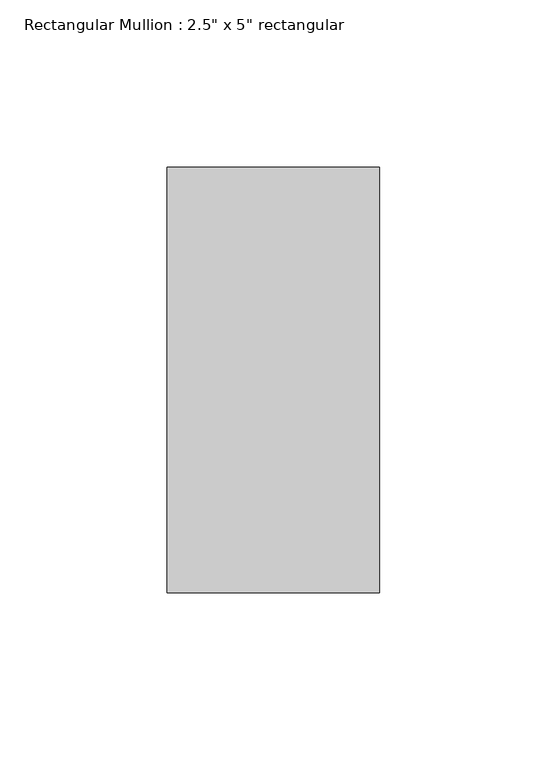
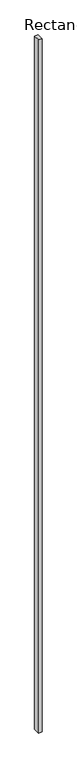
"""IFC4 building model written with IfcOpenShell, lengths in millimetres: member geometry."""

from ifc_helpers import new_model, si_unit, frame, origin, place, context, project, spatial, polyline, outline, extrude, source, transform, mapped, element, save


def member_ead6e1d0(model_context):
    return source(origin(), model_context, "Body", "SweptSolid", [
        extrude(outline(polyline([(0.0, 63.5), (0.0, -63.5), (-63.5, -63.5), (-63.5, 63.5), (0.0, 63.5)])), frame((0.0, 0.0, -13716.0), z_axis=(0.0, 0.0, 1.0), x_axis=(1.0, 0.0, 0.0)), (0.0, 0.0, 1.0), 13716.0),
    ])


if __name__ == "__main__":
    model = new_model("IFC4")
    model_context = context("Model", 3, world=origin())
    ifc_project = project(units=[si_unit("LENGTHUNIT", "METRE", prefix="MILLI")], contexts=[model_context])
    site = spatial("IfcSite", under=ifc_project)
    building = spatial("IfcBuilding", under=site)
    placement = place(None, origin())
    member_shape = member_ead6e1d0(model_context)
    element("IfcMember", 1, ObjectType="Rectangular Mullion : 2.5\" x 5\" rectangular", at=placement, inside=building, context=model_context, shape_type="MappedRepresentation", body=[
        mapped(member_shape, transform((0.0, 0.0, 0.0), x_axis=(1.0, 0.0, 0.0), y_axis=(0.0, 1.0, 0.0), z_axis=(0.0, 0.0, 1.0))),
    ])
    save(model, "model.ifc")

# Revit data of these elements
# Type "Rectangular Mullion : 2.5\" x 5\" rectangular"
#   built-in parameter 1007304 = 0.416667 (stored number, unit not read)
#   built-in parameter 1007301 = 0.104167 (stored number, unit not read)
#   built-in parameter 1007300 = 0.104167 (stored number, unit not read)
# Element 1 (IfcMember, "Rectangular Mullion : 2.5\" x 5\" rectangular")
#   Materials on its faces: "Aluminum"
# Materials
#   "Aluminum": class "Metal", colour RGB 247 247 247, transparency 0, Description = "Aluminum 6061", Cost = 0
